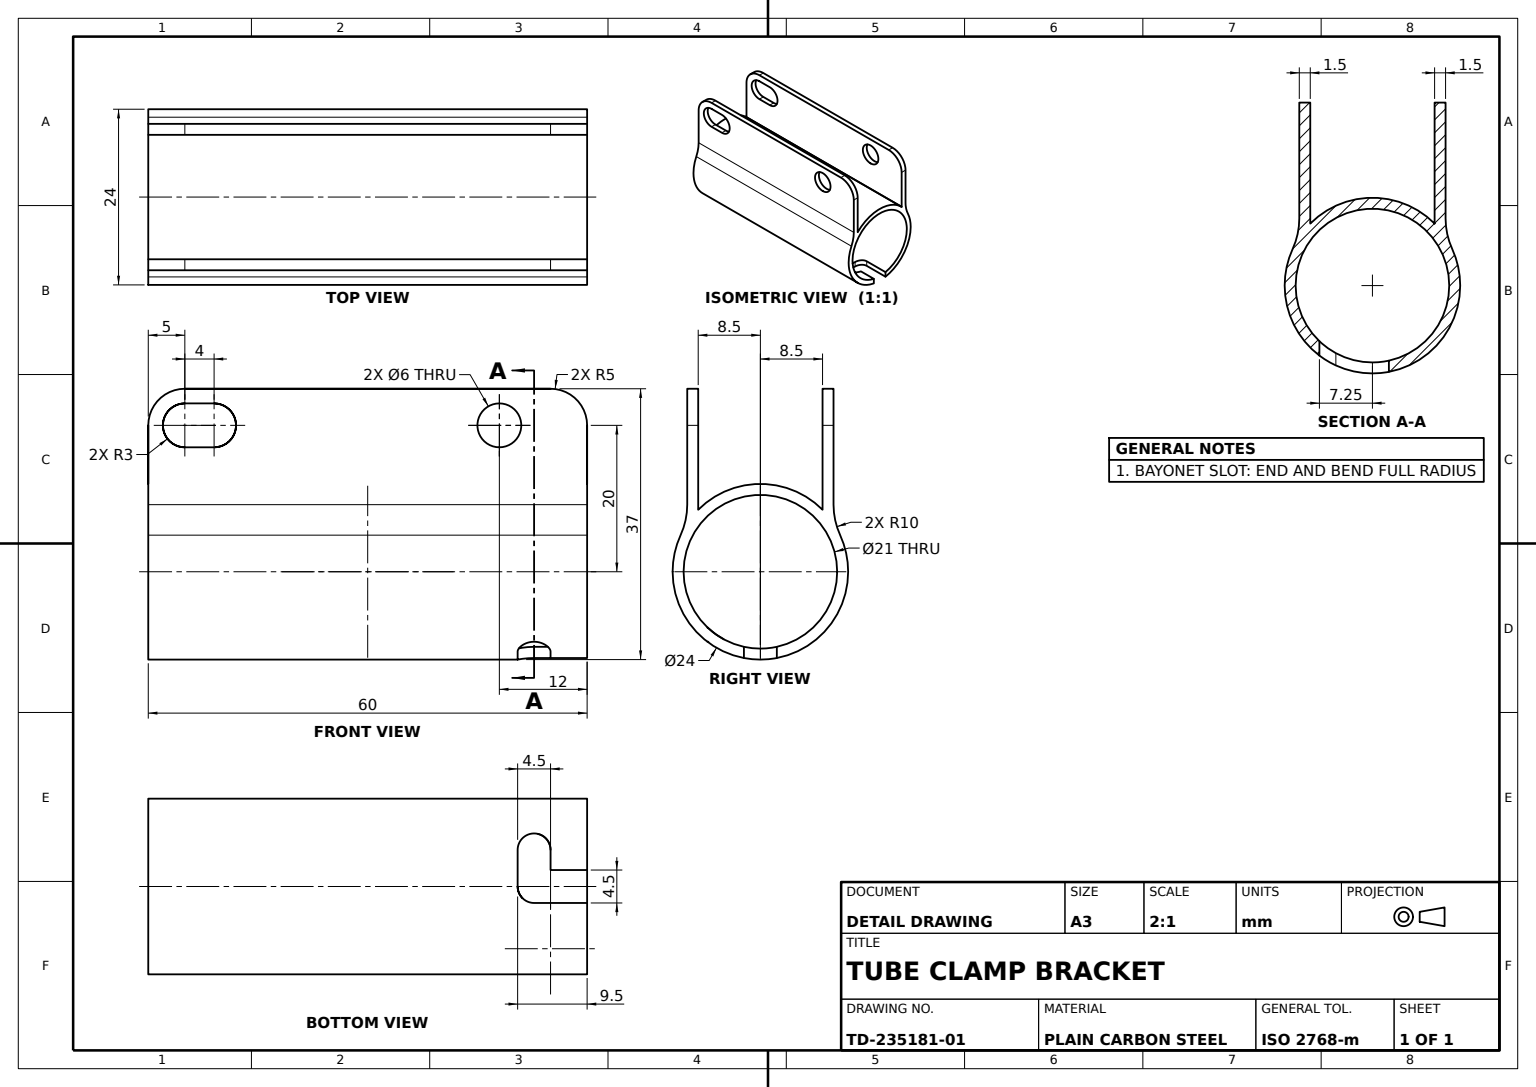
SolidWorks part; units mm, degrees
material "Plain Carbon Steel"
ref_plane "Front Plane" through (0, 0, 0) normal (0, 0, 1) x (1, 0, 0)
ref_plane "Top Plane" through (0, 0, 0) normal (0, 1, 0) x (1, 0, 0)
ref_plane "Right Plane" through (0, 0, 0) normal (1, 0, 0) x (0, 0, -1)
sketch "Sleeve Tube Profile" plane through (0, 0, 0) normal (0, 0, 1) x (1, 0, 0)
  circle A0 centre (0, 0) radius 12
  circle A1 centre (0, 0) radius 10.5
  dimension "D1" = 24
  dimension "D2" = 21
extrude "Sleeve Tube Ø24x60" add sketch "Sleeve Tube Profile" along normal mid plane 60
sketch "Mounting Lugs Profile" plane through (0, 0, 30) normal (0, 0, 1) x (1, 0, 0)
  line L0 (0, 0) -> (0, 22.8553) construction
  line L1 (-8.5, 25) -> (-8.5, 8.4705)
  line L2 (-10, 25) -> (-10, 6.6332)
  line L3 (-10, 25) -> (-8.5, 25)
  line L4 (10, 25) -> (10, 6.6332)
  line L5 (10, 25) -> (8.5, 25)
  line L6 (8.5, 25) -> (8.5, 8.4705)
  circle A0 centre (0, 0) radius 12 construction
  arc A1 (10, 6.6332) -> (8.5, 8.4705) centre (0, 0) ccw
  arc A2 (-8.5, 8.4705) -> (-10, 6.6332) centre (0, 0) ccw
  dimension "D1" = 8.5
  dimension "D2" = 1.5
  dimension "D3" = 25
extrude "Mounting Lugs" add sketch "Mounting Lugs Profile" against normal blind 60
fillet "Lug Fillet R10" radius 10 2 edges at (10, 6.6332, 0) (-10, 6.6332, 0)
fillet "Lug Fillet R5" radius 5 4 edges at (-9.25, 25, 30) (-9.25, 25, -30) (9.25, 25, 30) (9.25, 25, -30)
sketch "Lug Gap Cut Profile" plane through (10, 0, 0) normal (1, 0, 0) x (0, 0, -1)
  line L0 (-25, 20) -> (-21, 20) construction
  line L1 (-25, 23) -> (-21, 23)
  line L2 (-25, 17) -> (-21, 17)
  line L3 (-30, 4.9992) -> (-30, -12) construction
  line L4 (25, 25) -> (-25, 25) construction
  line L5 (30, 9.1652) -> (30, 20) construction
  arc A0 (-25, 23) -> (-25, 17) centre (-25, 20) ccw
  arc A1 (-21, 17) -> (-21, 23) centre (-21, 20) ccw
  circle A2 centre (18, 20) radius 3
  point P2 (-23, 20)
  dimension "D2" = 3
  dimension "D4" = 6
  dimension "D1" = 4
  dimension "D3" = 5
  dimension "D5" = 5
  dimension "D6" = 12
extrude "Lug Gap Cut" cut sketch "Lug Gap Cut Profile" against normal blind 60
sketch "Lug Slots Profile" plane through (0, 0, 0) normal (0, 1, 0) x (1, 0, 0)
  line L0 (-2.25, 30) -> (-2.25, 22.75)
  line L1 (12, 30) -> (-12, 30) construction
  line L2 (0, 20.5) -> (5, 20.5)
  line L3 (5, 25) -> (2.25, 25)
  line L4 (2.25, 25) -> (2.25, 30)
  line L5 (2.25, 30) -> (-2.25, 30)
  arc A0 (5, 20.5) -> (5, 25) centre (5, 22.75) ccw
  arc A1 (0, 20.5) -> (-2.25, 22.75) centre (0, 22.75) cw
  point P7 (7.25, 22.75)
  point P10 (0, 30)
  dimension "D5" = 2.25
  dimension "D1" = 4.5
  dimension "D2" = 5
  dimension "D3" = 4.5
  dimension "D4" = 5
extrude "Lug Slots" cut sketch "Lug Slots Profile" against normal up to surface (11.7872 mm away)
